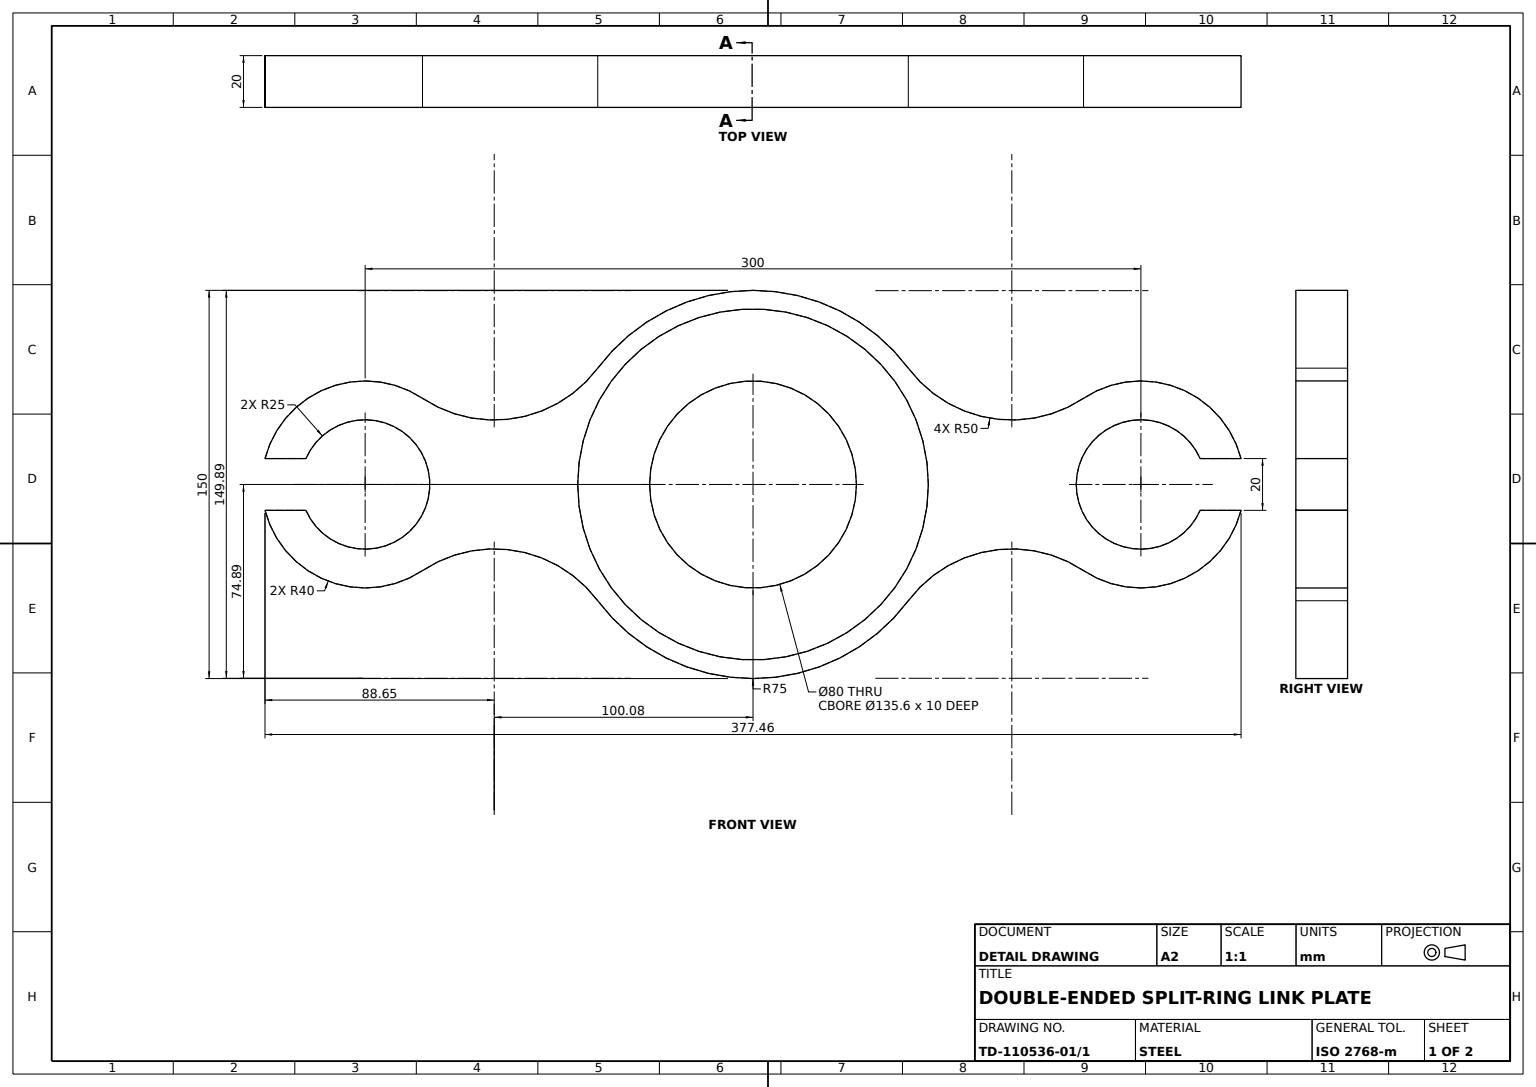
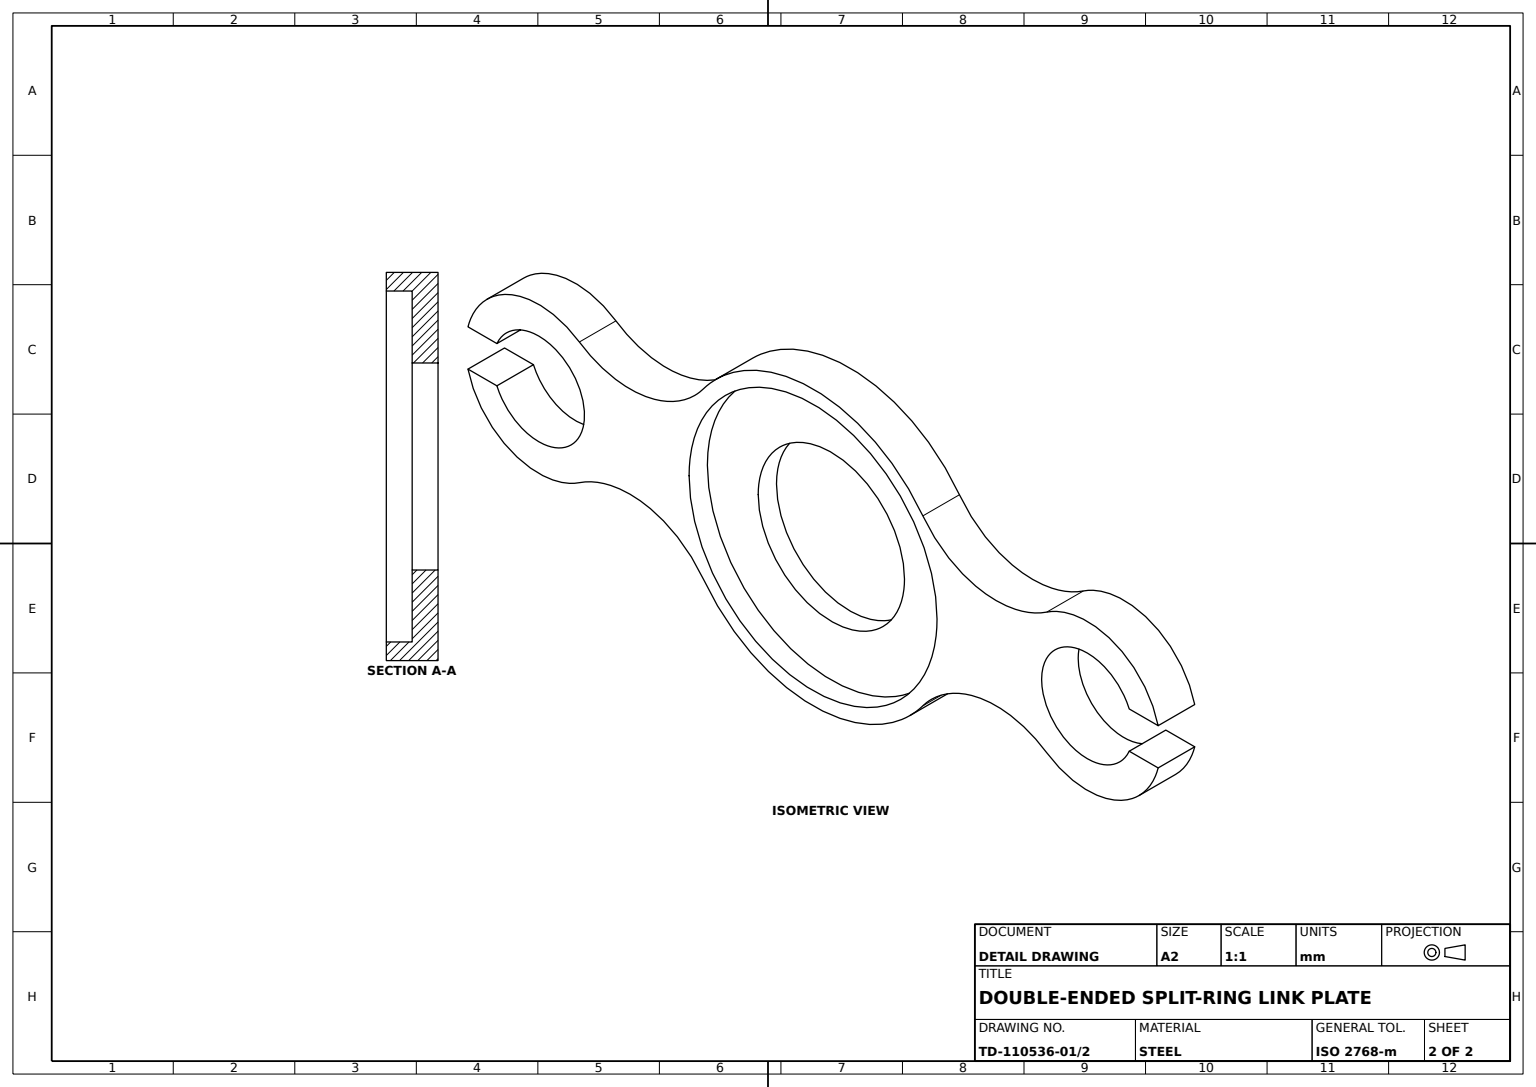
from build123d import *

# Parameters (mm, degrees)
LINK_PLATE_20MM_DEPTH       = 20
CENTRE_OPENING_SKETCH_R     = 67.8
CENTRE_OPENING_135_6_DEPTH  = 20
ANNULAR_WEB_SKETCH_R        = 67.8
ANNULAR_WEB_SKETCH_R_2      = 40
ANNULAR_WEB_80X_135_6_DEPTH = 10


with BuildPart() as part:
    # Link Plate Outline Sketch → Link Plate 20mm (new body)
    with BuildSketch(Plane.XY):
        with BuildLine():
            Line((-38.729833462, 10), (-22.912878475, 10))
            ThreePointArc((-22.912878475, 10), (25, 0), (-22.912878475, -10))
            Line((-22.912878475, -10), (-38.729833462, -10))
            ThreePointArc((-38.729833462, -10), (-14.281675999, -37.363534772), (22.185185185, -33.283893377))
            ThreePointArc((22.185185185, -33.283893377), (58.387841465, -25.611592996), (89.95, -44.933256058))
            ThreePointArc((89.95, -44.933256058), (150, -75), (210.05, -44.933256058))
            ThreePointArc((210.05, -44.933256058), (241.612158535, -25.611592996), (277.814814815, -33.283893377))
            ThreePointArc((277.814814815, -33.283893377), (314.281675999, -37.363534772), (338.729833462, -10))
            Line((338.729833462, -10), (322.912878475, -10))
            ThreePointArc((322.912878475, -10), (275, 0), (322.912878475, 10))
            Line((322.912878475, 10), (338.729833462, 10))
            ThreePointArc((338.729833462, 10), (314.281675999, 37.363534772), (277.814814815, 33.283893377))
            ThreePointArc((277.814814815, 33.283893377), (241.612158535, 25.611592996), (210.05, 44.933256058))
            ThreePointArc((210.05, 44.933256058), (150, 75), (89.95, 44.933256058))
            ThreePointArc((89.95, 44.933256058), (58.387841465, 25.611592996), (22.185185185, 33.283893377))
            ThreePointArc((22.185185185, 33.283893377), (-14.281675999, 37.363534772), (-38.729833462, 10))
        make_face()
    extrude(amount=LINK_PLATE_20MM_DEPTH)

    # Centre Opening Sketch → Centre Opening Ø135.6 (cut)
    with BuildSketch(Plane.XY.offset(20)):
        with Locations((150, 0)):
            Circle(CENTRE_OPENING_SKETCH_R)
    extrude(amount=-CENTRE_OPENING_135_6_DEPTH, mode=Mode.SUBTRACT)

    # Annular Web Sketch → Annular Web Ø80xØ135.6 (add)
    with BuildSketch(Plane.XY.offset(10)):
        with Locations((150, 0)):
            Circle(ANNULAR_WEB_SKETCH_R)
        with Locations((150, 0)):
            Circle(ANNULAR_WEB_SKETCH_R_2, mode=Mode.SUBTRACT)
    extrude(amount=-ANNULAR_WEB_80X_135_6_DEPTH)


solid = part.part
